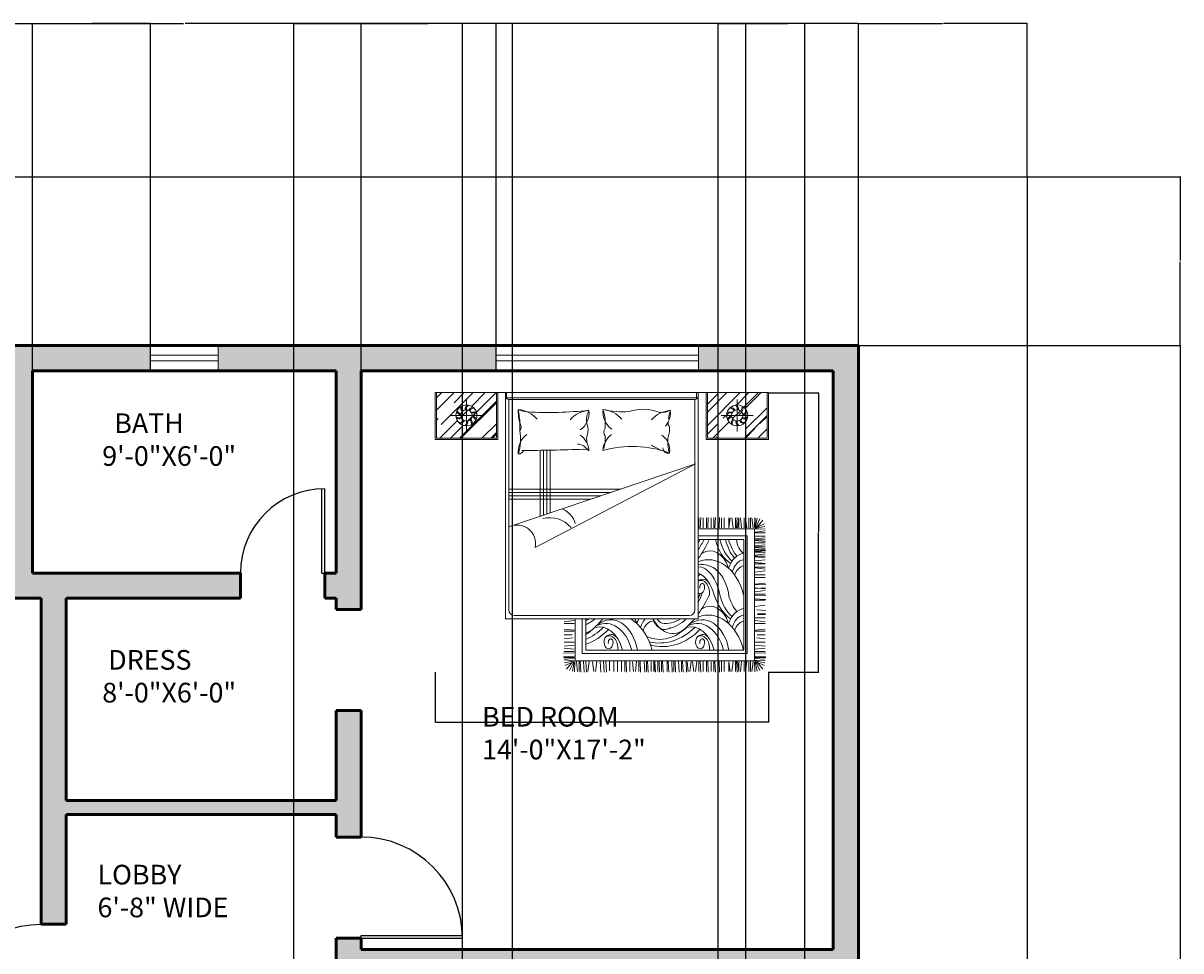
# Model space of a CAD drawing. Units: inches. Extents: x 134045 to 134755, y 144691 to 145880.
# Tile 6 of 6: x 134343 to 134755, y 145550 to 145880. Entities that reach past the tile are written whole.
import ezdxf

# ---------------------------------------------------------------- set-up
doc = ezdxf.new("R2010")
doc.units = ezdxf.units.IN
for name, color, linetype, lineweight in [('A-ANNO-DIMS', 2, 'Continuous', 18), ('A-AREA-IDEN', 7, 'Continuous', 18), ('A-DOOR', 4, 'Continuous', 25), ('A-FURN', 8, 'Continuous', 18), ('A-GLAZ', 4, 'Continuous', 18), ('A-WALL', 7, 'Continuous', 50), ('A-WALL-PATT', 252, 'Continuous', 13), ('C-PROP', 7, 'Continuous', 25)]:
    doc.layers.add(name, color=color, linetype=linetype, lineweight=lineweight)
doc.styles.get("Standard").update_dxf_attribs({"font": 'arial.ttf'})
doc.dimstyles.get("Standard").update_dxf_attribs({"dimtxt": 0.18, "dimasz": 0.18, "dimexe": 0.18, "dimexo": 0.0625, "dimgap": 0.09, "dimtad": 0, "dimtih": 1, "dimtoh": 1, "dimdec": 4, "dimzin": 0, "dimdsep": 46, "dimtxsty": 'Standard', "dimcen": 0.09, "dimadec": 0, "dimazin": 0, "dimtfac": 1, "dimtdec": 4, "dimtofl": 0, "dimtmove": 0, "dimatfit": 3, "dimfxl": 1, "dimtolj": 1, "dimtzin": 0, "dimarcsym": 0})

# ---------------------------------------------------------------- blocks, each defined once
blk = doc.blocks.new('A$C64B41DC1')
for p, q in [((0, 2.508), (2.99, 2.508)), ((0, 2.088), (0, 2.508)), ((0.012, 2.462), (0.058, 2.508)), ((0.012, 2.352), (0.168, 2.508)), ((0.012, 2.1), (0.012, 2.508)), ((0.054, 2.221), (0.341, 2.508)), ((0.169, 2.418), (0.259, 2.508)), ((0.327, 2.386), (0.448, 2.508)), ((0.37, 2.333), (0.545, 2.508)), ((0.548, 2.508), (0.548, 2.1)), ((0.56, 2.508), (0.56, 2.088)), ((0.63, 2.508), (0.63, 0.478)), ((0.64, 2.461), (0.64, 2.508)), ((0.64, 2.508), (2.344, 2.508)), ((2.344, 2.508), (2.36, 2.508)), ((2.344, 2.508), (2.344, 2.461)), ((2.36, 2.508), (2.36, 2.476)), ((2.36, 0.478), (2.36, 2.508)), ((2.43, 2.508), (2.43, 2.088)), ((2.442, 2.508), (2.442, 2.1)), ((2.442, 2.333), (2.617, 2.508)), ((2.442, 2.214), (2.736, 2.508)), ((2.442, 2.404), (2.535, 2.497)), ((2.705, 2.398), (2.815, 2.508)), ((2.769, 2.377), (2.9, 2.508)), ((2.782, 2.365), (2.925, 2.508)), ((2.978, 2.1), (2.978, 2.508)), ((2.99, 2.088), (2.99, 2.508)), ((0.216, 2.1), (0.548, 2.432)), ((0.23, 2.1), (0.548, 2.418)), ((0.28, 2.16), (0.28, 2.448)), ((2.344, 2.461), (0.64, 2.461)), ((0.66, 2.446), (1.495, 2.446)), ((0.66, 2.446), (0.66, 0.558)), ((1.495, 2.446), (0.67, 2.446)), ((2.33, 2.446), (1.495, 2.446)), ((2.33, 0.558), (2.33, 2.446)), ((2.71, 2.16), (2.71, 2.448)), ((0.136, 2.304), (0.425, 2.304)), ((0.231, 2.291), (0.294, 2.353)), ((0.291, 2.254), (0.33, 2.294)), ((0.341, 2.304), (0.36, 2.324)), ((2.854, 2.304), (2.566, 2.304)), ((2.585, 2.278), (2.616, 2.309)), ((2.616, 2.309), (2.631, 2.324)), ((2.667, 2.276), (2.738, 2.346)), ((2.725, 2.308), (2.751, 2.334)), ((2.775, 2.1), (2.978, 2.304)), ((2.791, 2.185), (2.978, 2.371)), ((2.914, 2.231), (2.978, 2.295)), ((0.012, 2.261), (0.027, 2.276)), ((0.04, 2.1), (0.198, 2.258)), ((0.137, 2.1), (0.251, 2.214)), ((0.419, 2.1), (0.548, 2.229)), ((2.442, 2.135), (2.538, 2.231)), ((2.492, 2.1), (2.637, 2.245)), ((2.783, 2.1), (2.868, 2.185)), ((0.56, 2.088), (0, 2.088)), ((0.548, 2.1), (0.012, 2.1)), ((0.499, 2.1), (0.548, 2.149)), ((0.513, 2.1), (0.548, 2.135)), ((2.43, 2.088), (2.99, 2.088)), ((2.442, 2.1), (2.978, 2.1)), ((2.517, 2.1), (2.527, 2.11)), ((2.896, 2.1), (2.978, 2.182)), ((0.942, 1.99), (0.942, 1.397)), ((0.972, 1.991), (0.972, 1.408)), ((1.002, 1.991), (1.002, 1.418)), ((1.032, 1.992), (1.032, 1.428)), ((2.335, 1.868), (0.661, 1.303)), ((0.896, 1.119), (2.335, 1.868)), ((1.664, 1.641), (0.66, 1.641)), ((1.575, 1.611), (0.66, 1.611)), ((2.366, 1.295), (2.366, 1.384)), ((2.377, 1.295), (2.382, 1.389)), ((2.403, 1.295), (2.403, 1.384)), ((2.435, 1.295), (2.435, 1.384)), ((2.445, 1.295), (2.45, 1.389)), ((2.477, 1.296), (2.477, 1.384)), ((2.5, 1.295), (2.5, 1.384)), ((2.51, 1.295), (2.516, 1.389)), ((2.537, 1.295), (2.537, 1.384)), ((2.547, 1.295), (2.552, 1.389)), ((2.568, 1.295), (2.568, 1.384)), ((2.592, 1.295), (2.592, 1.384)), ((2.635, 1.296), (2.635, 1.384)), ((2.636, 1.296), (2.647, 1.384)), ((2.673, 1.295), (2.662, 1.384)), ((2.694, 1.295), (2.694, 1.384)), ((2.704, 1.295), (2.71, 1.389)), ((2.713, 1.296), (2.723, 1.384)), ((2.725, 1.295), (2.725, 1.384)), ((2.749, 1.295), (2.739, 1.384)), ((2.772, 1.295), (2.772, 1.384)), ((2.796, 1.295), (2.785, 1.384)), ((2.815, 1.296), (2.815, 1.384)), ((2.815, 1.296), (2.815, 1.384)), ((2.828, 1.295), (2.828, 1.384)), ((2.828, 1.295), (2.828, 1.384)), ((2.852, 1.295), (2.842, 1.384)), ((2.852, 1.295), (2.842, 1.384)), ((2.865, 1.297), (2.869, 1.386)), ((2.871, 1.296), (2.871, 1.384)), ((2.871, 1.296), (2.888, 1.382)), ((2.877, 1.296), (2.913, 1.376)), ((2.889, 1.301), (2.939, 1.364)), ((2.36, 1.287), (2.864, 1.287)), ((2.864, 1.287), (2.864, 0.102)), ((2.871, 1.293), (2.954, 1.332)), ((2.872, 1.288), (2.959, 1.306)), ((2.872, 1.256), (2.96, 1.267)), ((2.872, 1.249), (2.96, 1.249)), ((2.874, 1.282), (2.96, 1.287)), ((2.36, 1.223), (2.8, 1.223)), ((2.36, 1.191), (2.768, 1.191)), ((2.768, 1.191), (2.768, 0.198)), ((2.8, 1.223), (2.8, 0.166)), ((2.872, 1.221), (2.96, 1.221)), ((2.872, 1.195), (2.96, 1.205)), ((2.872, 1.187), (2.96, 1.187)), ((2.872, 1.181), (2.96, 1.171)), ((2.872, 1.159), (2.96, 1.159)), ((2.872, 1.133), (2.96, 1.143)), ((2.872, 1.125), (2.96, 1.125)), ((2.872, 1.119), (2.96, 1.109)), ((2.872, 1.104), (2.96, 1.093)), ((2.872, 1.097), (2.96, 1.097)), ((2.872, 1.086), (2.966, 1.091)), ((2.872, 1.086), (2.96, 1.075)), ((2.872, 1.076), (2.96, 1.076)), ((2.872, 1.049), (2.96, 1.06)), ((2.872, 1.042), (2.96, 1.042)), ((2.872, 1.035), (2.96, 1.025)), ((2.872, 0.999), (2.96, 1.009)), ((2.872, 0.985), (2.96, 0.974)), ((2.872, 0.973), (2.96, 0.973)), ((2.872, 0.941), (2.96, 0.941)), ((2.872, 0.935), (2.96, 0.924)), ((2.872, 0.898), (2.96, 0.908)), ((2.872, 0.873), (2.96, 0.873)), ((2.872, 0.85), (2.96, 0.85)), ((2.872, 0.789), (2.96, 0.799)), ((2.872, 0.782), (2.966, 0.787)), ((2.872, 0.757), (2.96, 0.747)), ((2.872, 0.75), (2.966, 0.756)), ((2.872, 0.72), (2.96, 0.731)), ((2.872, 0.699), (2.96, 0.699)), ((2.872, 0.689), (2.966, 0.684)), ((2.872, 0.658), (2.966, 0.652)), ((2.872, 0.647), (2.96, 0.647)), ((2.872, 0.59), (2.96, 0.601)), ((2.882, 0.558), (2.966, 0.554)), ((2.891, 0.526), (2.966, 0.522)), ((0.63, 0.478), (2.36, 0.478)), ((0.71, 0.508), (2.28, 0.508)), ((1.246, 0.463), (1.158, 0.452)), ((1.246, 0.437), (1.158, 0.437)), ((1.254, 0.102), (1.254, 0.478)), ((1.318, 0.166), (1.318, 0.478)), ((1.35, 0.198), (1.35, 0.478)), ((2.872, 0.488), (2.96, 0.488)), ((2.872, 0.463), (2.96, 0.452)), ((2.872, 0.437), (2.96, 0.437)), ((2.893, 0.517), (2.96, 0.517)), ((1.246, 0.375), (1.158, 0.385)), ((1.246, 0.368), (1.158, 0.368)), ((1.229, 0.336), (1.158, 0.336)), ((2.872, 0.375), (2.96, 0.385)), ((2.872, 0.368), (2.96, 0.368)), ((2.89, 0.336), (2.96, 0.336)), ((1.235, 0.309), (1.158, 0.3)), ((1.246, 0.268), (1.158, 0.268)), ((1.246, 0.242), (1.158, 0.232)), ((1.246, 0.206), (1.158, 0.216)), ((2.872, 0.268), (2.96, 0.268)), ((2.872, 0.242), (2.96, 0.232)), ((2.872, 0.206), (2.96, 0.216)), ((2.883, 0.309), (2.96, 0.3)), ((1.246, 0.174), (1.152, 0.169)), ((1.246, 0.143), (1.152, 0.138)), ((1.246, 0.133), (1.152, 0.128)), ((1.246, 0.185), (1.158, 0.185)), ((1.246, 0.132), (1.158, 0.132)), ((1.246, 0.132), (1.158, 0.132)), ((1.246, 0.1), (1.158, 0.11)), ((1.246, 0.123), (1.159, 0.117)), ((2.8, 0.166), (1.318, 0.166)), ((2.768, 0.198), (1.35, 0.198)), ((2.872, 0.185), (2.96, 0.185)), ((2.872, 0.174), (2.966, 0.169)), ((2.872, 0.143), (2.966, 0.138)), ((2.872, 0.133), (2.966, 0.128)), ((2.872, 0.132), (2.96, 0.132)), ((2.872, 0.123), (2.959, 0.117)), ((2.874, 0.107), (2.96, 0.102)), ((1.246, 0.101), (1.159, 0.083)), ((1.247, 0.096), (1.164, 0.058)), ((1.229, 0.088), (1.179, 0.026)), ((1.242, 0.093), (1.205, 0.013)), ((1.247, 0.093), (1.231, 0.007)), ((1.253, 0.092), (1.249, 0.003)), ((2.864, 0.102), (1.254, 0.102)), ((1.266, 0.094), (1.276, 0.005)), ((1.29, 0.094), (1.29, 0.005)), ((1.3, 0.094), (1.305, 0)), ((1.331, 0.094), (1.337, 0)), ((1.352, 0.094), (1.358, 0)), ((1.38, 0.094), (1.37, 0.005)), ((1.412, 0.093), (1.422, 0.005)), ((1.449, 0.094), (1.438, 0.005)), ((1.48, 0.094), (1.485, 0)), ((1.511, 0.094), (1.517, 0)), ((1.532, 0.094), (1.538, 0)), ((1.564, 0.094), (1.564, 0.01)), ((1.602, 0.094), (1.602, 0.005)), ((1.634, 0.094), (1.634, 0.005)), ((1.67, 0.094), (1.67, 0.005)), ((1.702, 0.094), (1.702, 0.005)), ((1.712, 0.094), (1.717, 0)), ((1.745, 0.093), (1.745, 0.005)), ((1.77, 0.093), (1.78, 0.005)), ((1.806, 0.094), (1.796, 0.005)), ((1.827, 0.094), (1.827, 0.005)), ((1.838, 0.094), (1.843, 0)), ((1.875, 0.094), (1.88, 0)), ((1.896, 0.094), (1.896, 0.005)), ((1.906, 0.094), (1.911, 0)), ((1.938, 0.093), (1.938, 0.005)), ((1.961, 0.094), (1.961, 0.005)), ((1.964, 0.093), (1.974, 0.005)), ((1.971, 0.094), (1.977, 0)), ((1.998, 0.094), (1.998, 0.005)), ((2.008, 0.094), (2.013, 0)), ((2.029, 0.094), (2.029, 0.005)), ((2.039, 0.094), (2.045, 0)), ((2.08, 0.094), (2.08, 0.005)), ((2.09, 0.094), (2.095, 0)), ((2.122, 0.094), (2.127, 0)), ((2.141, 0.094), (2.141, 0.005)), ((2.152, 0.094), (2.157, 0)), ((2.183, 0.094), (2.188, 0)), ((2.209, 0.094), (2.209, 0.005)), ((2.22, 0.094), (2.225, 0)), ((2.251, 0.094), (2.256, 0)), ((2.26, 0.093), (2.271, 0.005)), ((2.297, 0.094), (2.286, 0.005)), ((2.309, 0.093), (2.319, 0.005)), ((2.346, 0.094), (2.335, 0.005)), ((2.366, 0.094), (2.366, 0.005)), ((2.377, 0.094), (2.382, 0)), ((2.403, 0.094), (2.403, 0.005)), ((2.435, 0.094), (2.435, 0.005)), ((2.445, 0.094), (2.45, 0)), ((2.477, 0.093), (2.477, 0.005)), ((2.5, 0.094), (2.5, 0.005)), ((2.51, 0.094), (2.516, 0)), ((2.537, 0.094), (2.537, 0.005)), ((2.547, 0.094), (2.552, 0)), ((2.568, 0.094), (2.568, 0.005)), ((2.592, 0.094), (2.592, 0.005)), ((2.635, 0.093), (2.635, 0.005)), ((2.636, 0.093), (2.647, 0.005)), ((2.673, 0.094), (2.662, 0.005)), ((2.694, 0.094), (2.694, 0.005)), ((2.704, 0.094), (2.71, 0)), ((2.713, 0.093), (2.723, 0.005)), ((2.725, 0.094), (2.725, 0.005)), ((2.749, 0.094), (2.739, 0.005)), ((2.772, 0.094), (2.772, 0.005)), ((2.796, 0.094), (2.785, 0.005)), ((2.815, 0.093), (2.815, 0.005)), ((2.828, 0.094), (2.828, 0.005)), ((2.852, 0.094), (2.842, 0.005)), ((2.865, 0.092), (2.869, 0.003)), ((2.871, 0.096), (2.954, 0.058)), ((2.871, 0.093), (2.888, 0.007)), ((2.872, 0.101), (2.959, 0.083)), ((2.877, 0.093), (2.913, 0.013)), ((2.889, 0.088), (2.939, 0.026))]:
    blk.add_line(p, q)
at = {"ltscale": 10}
for p, q in [((1.486, 1.581), (0.66, 1.581)), ((1.397, 1.551), (0.66, 1.551))]:
    blk.add_line(p, q, dxfattribs=at)
for centre, radius in [((0.28, 2.304), 0.0942), ((2.71, 2.304), 0.0942), ((0.28, 2.304), 0.051), ((2.71, 2.304), 0.051)]:
    blk.add_circle(centre, radius)
for centre, radius, start, end in [((0.329, 2.356), 0.0605, 136.17, 182.4897), ((0.323, 2.358), 0.0462, 124.3002, 184.538), ((0.66, 2.476), 0.03, 180, 270), ((2.33, 2.476), 0.03, 270, 0), ((2.667, 2.358), 0.0462, 355.462, 55.6998), ((2.662, 2.356), 0.0605, 357.5103, 43.83), ((0.215, 2.328), 0.0462, 232.3002, 292.538), ((0.246, 2.366), 0.0605, 208.17, 254.4897), ((0.242, 2.361), 0.0462, 196.3002, 256.538), ((0.289, 2.374), 0.0605, 172.17, 218.4897), ((0.283, 2.373), 0.0462, 160.3002, 220.538), ((0.35, 2.318), 0.0605, 100.17, 146.4897), ((0.347, 2.323), 0.0462, 88.3002, 148.538), ((0.345, 2.274), 0.0605, 64.17, 110.4897), ((0.345, 2.28), 0.0462, 52.3002, 112.538), ((0.319, 2.246), 0.0462, 16.3002, 76.538), ((0.315, 2.242), 0.0605, 28.17, 74.4897), ((1.053, 2.33), 0.308, 175.3048, 198.6942), ((-0.87, 2.094), 1.636, 4.8098, 9.1892), ((0.858, 2.628), 0.295, 247.5179, 264.267), ((0.728, 2.111), 0.245, 40.4189, 85.9871), ((1.016, 5.71), 3.38, 266.8134, 276.1602), ((1.396, 2.104), 0.245, 94.0129, 139.5811), ((1.186, 2.329), 0.194, 306.5711, 5.89), ((1.535, 2.265), 0.177, 151.7736, 201.6983), ((1.699, 2.335), 0.194, 174.11, 233.4289), ((1.148, 2.231), 0.378, 353.4947, 19.1867), ((1.687, 3.192), 0.856, 257.7438, 273.6284), ((1.488, 2.111), 0.245, 40.4189, 85.9871), ((1.867, 1.971), 0.388, 68.2026, 108.9817), ((2.127, 2.104), 0.245, 94.0129, 139.5811), ((2.034, 2.486), 0.156, 261.5958, 298.9092), ((1.916, 2.329), 0.194, 333.7371, 5.89), ((2.606, 2.203), 0.517, 163.6046, 172.3273), ((2.645, 2.28), 0.0462, 67.462, 127.6998), ((2.645, 2.274), 0.0605, 69.5103, 115.83), ((2.675, 2.242), 0.0605, 105.5103, 151.83), ((2.671, 2.246), 0.0462, 103.462, 163.6998), ((2.643, 2.323), 0.0462, 31.462, 91.6998), ((2.64, 2.318), 0.0605, 33.5103, 79.83), ((2.707, 2.373), 0.0462, 319.462, 19.6998), ((2.702, 2.374), 0.0605, 321.5103, 7.83), ((2.775, 2.328), 0.0462, 247.462, 307.6998), ((2.749, 2.361), 0.0462, 283.462, 343.6998), ((2.745, 2.366), 0.0605, 285.5103, 331.83), ((0.216, 2.334), 0.0605, 244.17, 290.4897), ((0.214, 2.285), 0.0462, 268.3002, 328.538), ((0.211, 2.29), 0.0605, 280.17, 326.4897), ((0.238, 2.249), 0.0462, 304.3002, 4.538), ((0.232, 2.252), 0.0605, 316.17, 2.4897), ((0.278, 2.235), 0.0462, 340.3002, 40.538), ((0.272, 2.233), 0.0605, 352.17, 38.4897), ((0.727, 2.201), 0.0446, 314.4736, 42.1713), ((-1.601, 2.277), 2.362, 357.3905, 358.8876), ((1.204, 2.178), 0.168, 337.017, 7.5368), ((1.567, 2.155), 0.0547, 142.0833, 220.902), ((1.916, 2.329), 0.194, 320.9404, 333.7371), ((2.135, 2.231), 0.0459, 165.3506, 223.2684), ((1.935, 2.178), 0.168, 337.017, 7.5368), ((2.718, 2.233), 0.0605, 141.5103, 187.83), ((2.712, 2.235), 0.0462, 139.462, 199.6998), ((2.758, 2.252), 0.0605, 177.5103, 223.83), ((2.753, 2.249), 0.0462, 175.462, 235.6998), ((2.78, 2.29), 0.0605, 213.5103, 259.83), ((2.777, 2.285), 0.0462, 211.462, 271.6998), ((2.774, 2.334), 0.0605, 249.5103, 295.83), ((0.938, 1.978), 0.194, 126.5711, 185.89), ((0.269, 2.094), 0.496, 344.0243, 8.7071), ((1.186, 1.971), 0.194, 4.3181, 53.4289), ((1.541, 2.097), 0.183, 175.2233, 196.23), ((1.706, 1.971), 0.204, 127.1197, 175.09), ((1.196, 2.098), 0.33, 343.7954, 3.5554), ((1.939, 1.991), 0.165, 351.2621, 55.7572), ((2.462, 2.072), 0.375, 173.8296, 196.4356), ((0.742, 2.015), 0.057, 273.4709, 328.5412), ((0.725, 18.844), 16.855, 270.174, 272.0521), ((1.269, 1.925), 0.122, 33.628, 86.4744), ((1.34, 1.94), 0.0603, 49.0991, 101.3702), ((1.768, 1.063), 0.963, 69.6507, 105.9631), ((2.275, 2.579), 0.637, 238.3499, 254.3137), ((2.091, 2.012), 0.0478, 179.7727, 283.8018), ((0.728, 2.202), 0.245, 274.0129, 278.3417), ((1.075, 1.287), 0.187, 14.1863, 69.1212), ((1.027, 1.133), 0.253, 40.629, 104.3712), ((0.735, 1.155), 0.165, 347.3109, 116.4454), ((0.71, 0.558), 0.05, 180, 270), ((2.28, 0.558), 0.05, 270, 0)]:
    blk.add_arc(centre, radius, start, end)
for centre, major_axis, ratio, start_param, end_param in [((1.994, 1.626), (0, -0.753), 0.68, 0.797284, 0.954936), ((2.064, 1.466), (0, -0.532), 0.68, 7.239912, 7.311536), ((1.905, 1.74), (0, -0.984), 0.68, 0.74745, 0.979724), ((2.746, 1.308), (0, 0.361), 0.68, 1.900046, 2.742661), ((2.787, 1.308), (0, 0.361), 0.68, 1.900046, 2.614747), ((2.837, 1.308), (0, 0.361), 0.68, 1.900046, 2.479658), ((2.861, 1.321), (0, 0.361), 0.68, 1.938265, 2.479658), ((2.806, 1.208), (0, -0.152), 0.68, 4.821745, 5.895886), ((2.451, 0.507), (0, 0.502), 0.68, 5.095327, 6.553458), ((2.467, 0.822), (0, -0.266), 0.68, 2.006169, 3.565187), ((2.786, 0.807), (0, -0.261), 0.68, 3.244645, 4.205018), ((2.396, 0.603), (0, 0.364), 0.68, -1.3172, 0.145284), ((2.351, 0.564), (0.007, 0.382), 0.56205, -1.21172, -0.009991), ((2.778, 0.829), (0, -0.18), 0.68, 3.227058, 4.318474), ((2.782, 0.797), (0, -0.159), 0.68, 3.272942, 4.229533), ((2.296, 0.577), (0, -0.326), 0.68, 1.938944, 2.850232), ((2.04, 1.601), (0, -0.876), 0.68, 6.849801, 6.887077), ((2.4, 0.713), (0, -0.121), 0.68, 2.284368, 3.652258), ((2.383, 0.708), (0, 0.115), 0.68, 4.593909, 6.585576), ((2.377, 0.765), (0, -0.0593), 0.68, 5.841311, 7.755362), ((2.396, 0.763), (0, -0.0317), 0.68, 1.462497, 5.046281), ((1.994, 1.13), (-0.068, 0.744), 0.610498, 3.917146, 4.063997), ((2.064, 0.969), (0, -0.532), 0.68, 7.239912, 7.336618), ((1.905, 1.243), (0, -0.984), 0.68, 0.74745, 0.979724), ((2.467, 0.325), (0, -0.266), 0.68, 2.006169, 3.565187), ((2.746, 0.811), (-0.06, 0.373), 0.695517, 1.775813, 2.548612), ((2.787, 0.811), (0, 0.361), 0.68, 1.900046, 2.614747), ((2.861, 0.824), (0, 0.361), 0.68, 1.938265, 2.479658), ((2.451, 0.01), (0, 0.502), 0.68, 5.095327, 6.553458), ((2.786, 0.31), (0, -0.261), 0.68, 3.244645, 4.205018), ((1.242, 0.969), (0, -0.532), 0.68, 6.586764, 6.677612), ((1.171, 1.13), (-0.116, 0.724), 0.59432, 3.291697, 3.50733), ((1.474, 0.08), (0, -0.326), 0.68, 1.938944, 3.339184), ((1.083, 1.243), (0, -0.984), 0.68, 0.565948, 0.680366), ((1.528, 0.067), (0, -0.37), 0.68, 1.930561, 3.464283), ((1.574, 0.106), (0, 0.364), 0.68, -1.3172, 0.476403), ((1.629, 0.01), (0, 0.502), 0.68, 6.655152, 6.661293), ((1.629, 0.01), (0, 0.502), 0.68, 5.095327, 5.911219), ((1.644, 0.325), (0, -0.266), 0.68, 2.006169, 2.182797), ((1.964, 0.31), (0, -0.261), 0.68, 4.015924, 4.205018), ((1.956, 0.332), (0, -0.18), 0.68, 3.770744, 4.318474), ((1.96, 0.3), (0, -0.159), 0.68, 3.14258, 4.229533), ((2.061, 0.562), (0, -0.18), 0.68, 5.194792, 5.929328), ((2.061, 0.562), (0, -0.18), 0.68, 5.194792, 6.723255), ((2.131, 0.66), (0, -0.315), 0.68, 5.328638, 6.949396), ((2.055, 0.566), (0, -0.13), 0.68, 5.450951, 6.054641), ((2.064, 0.969), (0, -0.532), 0.68, 6.20013, 6.677612), ((1.994, 1.13), (-0.068, 0.744), 0.610498, 3.199135, 3.592282), ((2.296, 0.08), (0, -0.326), 0.68, 1.938944, 3.339184), ((1.905, 1.243), (0, -0.984), 0.68, 0.565948, 0.680366), ((2.351, 0.067), (0, -0.37), 0.68, 1.930561, 3.464283), ((2.396, 0.106), (0, 0.364), 0.68, -1.3172, 0.476403), ((2.451, 0.01), (0, 0.502), 0.68, 6.655152, 6.661293), ((2.778, 0.332), (0, -0.18), 0.68, 3.227058, 4.318474), ((2.782, 0.3), (0, -0.159), 0.68, 3.272942, 4.229533), ((1.193, 0.918), (0, -0.624), 0.68, 0.378672, 0.625379), ((1.309, 0.66), (0, -0.315), 0.68, 6.475719, 6.949396), ((1.191, 1.107), (0, 0.846), 0.68, 3.421828, 3.728616), ((1.218, 1.105), (0, -0.876), 0.68, 6.507006, 6.887077), ((1.555, 0.269), (0, -0.0593), 0.68, 3.732151, 7.755362), ((1.578, 0.217), (0, -0.121), 0.68, 2.284368, 3.726131), ((1.561, 0.211), (0, 0.115), 0.68, 4.593909, 6.647252), ((2.016, 0.918), (0, -0.624), 0.68, -0.280078, 0.625379), ((2.013, 1.107), (0, 0.846), 0.68, 2.978727, 3.728616), ((2.04, 1.105), (0, -0.876), 0.68, 6.099302, 6.887077), ((2.377, 0.269), (0, -0.0593), 0.68, 3.732151, 7.755362), ((2.4, 0.217), (0, -0.121), 0.68, 2.284368, 3.726131), ((2.383, 0.211), (0, 0.115), 0.68, 4.593909, 6.647252), ((1.574, 0.266), (0, -0.0317), 0.68, 1.462497, 5.046281), ((2.396, 0.266), (0, -0.0317), 0.68, 1.462497, 5.046281)]:
    blk.add_ellipse(centre, major_axis=major_axis, ratio=ratio, start_param=start_param, end_param=end_param)
blk = doc.blocks.new('DOOR-SWING-36IN')
for p, q in [((0, 1), (35.99, 1)), ((0, 0), (0, 1)), ((0, 0), (36, 0))]:
    blk.add_line(p, q)
blk.add_arc((0, 0), 36, 0, 90)
blk = doc.blocks.new('DOOR-SWING-30IN')
for p, q in [((0, 1), (29.98, 1)), ((0, 1), (0, 0)), ((0, 0), (30, 0))]:
    blk.add_line(p, q)
blk.add_arc((0, 0), 30, 0, 90)
blk = doc.blocks.new('WIN-GLAZ-24IN')
for p, q in [((0, 0), (0, 24)), ((2, 0), (2, 24))]:
    blk.add_line(p, q)
blk = doc.blocks.new('WIN-GLAZ-72IN')
for p, q in [((0, 72), (0, 0)), ((2, 72), (2, 0))]:
    blk.add_line(p, q)
blk = doc.blocks.new('*D32')
at = {"layer": 'A-ANNO-DIMS', "color": 0, "lineweight": -2, "transparency": 16777216}
for p, q in [((134489.45, 145649.04), (134489.45, 145631.13)), ((134608.05, 145649.04), (134608.05, 145631.13)), ((134489.63, 145631.31), (134547.37, 145631.31)), ((134607.87, 145631.31), (134550.14, 145631.31))]:
    blk.add_line(p, q, dxfattribs=at)
at = {"layer": 'A-ANNO-DIMS', "color": 0, "transparency": 16777216}
for points in [[(134489.63, 145631.34), (134489.63, 145631.28), (134489.45, 145631.31)], [(134607.87, 145631.34), (134607.87, 145631.28), (134608.05, 145631.31)]]:
    blk.add_solid(points, dxfattribs=at)
at = {"layer": 'Defpoints', "color": 0, "transparency": 16777216}
for p in [(134489.45, 145649.1), (134608.05, 145649.1), (134608.05, 145631.31)]:
    blk.add_point(p, dxfattribs=at)
at = {"layer": 'A-ANNO-DIMS', "color": 0, "transparency": 16777216, "insert": (134548.75, 145631.31), "char_height": 0.18, "attachment_point": 5}
blk.add_mtext('\\A1;BED GROUP 119 TYP.', dxfattribs=at)
blk = doc.blocks.new('*D33')
at = {"layer": 'A-ANNO-DIMS', "color": 0, "lineweight": -2, "transparency": 16777216}
for p, q in [((134608.12, 145748.57), (134626.03, 145748.57)), ((134625.85, 145748.39), (134625.85, 145699.02)), ((134625.85, 145649.28), (134625.85, 145698.65)), ((134608.12, 145649.1), (134626.03, 145649.1))]:
    blk.add_line(p, q, dxfattribs=at)
at = {"layer": 'A-ANNO-DIMS', "color": 0, "transparency": 16777216}
for points in [[(134625.82, 145748.39), (134625.88, 145748.39), (134625.85, 145748.57)], [(134625.82, 145649.28), (134625.88, 145649.28), (134625.85, 145649.1)]]:
    blk.add_solid(points, dxfattribs=at)
at = {"layer": 'Defpoints', "color": 0, "transparency": 16777216}
for p in [(134608.05, 145748.57), (134625.85, 145748.57), (134608.05, 145649.1)]:
    blk.add_point(p, dxfattribs=at)
at = {"layer": 'A-ANNO-DIMS', "color": 0, "transparency": 16777216, "insert": (134625.85, 145698.83), "char_height": 0.18, "attachment_point": 5}
blk.add_mtext('\\A1;99 TYP.', dxfattribs=at)
blk = doc.blocks.new('*D48')
at = {"layer": 'A-ANNO-DIMS', "color": 0, "lineweight": -2, "transparency": 16777216}
for p, q in [((134160.1, 145765.44), (134160.1, 145880.11)), ((134160.28, 145879.93), (134399.81, 145879.93)), ((134639.92, 145879.93), (134400.4, 145879.93)), ((134640.1, 145765.44), (134640.1, 145880.11))]:
    blk.add_line(p, q, dxfattribs=at)
at = {"layer": 'A-ANNO-DIMS', "color": 0, "transparency": 16777216}
for points in [[(134160.28, 145879.96), (134160.28, 145879.9), (134160.1, 145879.93)], [(134639.92, 145879.96), (134639.92, 145879.9), (134640.1, 145879.93)]]:
    blk.add_solid(points, dxfattribs=at)
at = {"layer": 'Defpoints', "color": 0, "transparency": 16777216}
for p in [(134640.1, 145879.93), (134160.1, 145765.38), (134640.1, 145765.38)]:
    blk.add_point(p, dxfattribs=at)
at = {"layer": 'A-ANNO-DIMS', "color": 0, "transparency": 16777216, "insert": (134400.1, 145879.93), "char_height": 0.18, "attachment_point": 5}
blk.add_mtext('\\A1;480', dxfattribs=at)
blk = doc.blocks.new('*D49')
at = {"layer": 'A-ANNO-DIMS', "color": 0, "lineweight": -2, "transparency": 16777216}
for p, q in [((134640.17, 145765.38), (134754.83, 145765.38)), ((134754.65, 145765.2), (134754.65, 145358.06)), ((134754.65, 144950.56), (134754.65, 145357.69)), ((134640.17, 144950.38), (134754.83, 144950.38))]:
    blk.add_line(p, q, dxfattribs=at)
at = {"layer": 'A-ANNO-DIMS', "color": 0, "transparency": 16777216}
for points in [[(134754.62, 145765.2), (134754.68, 145765.2), (134754.65, 145765.38)], [(134754.62, 144950.56), (134754.68, 144950.56), (134754.65, 144950.38)]]:
    blk.add_solid(points, dxfattribs=at)
at = {"layer": 'Defpoints', "color": 0, "transparency": 16777216}
for p in [(134640.1, 145765.38), (134754.65, 145765.38), (134640.1, 144950.38)]:
    blk.add_point(p, dxfattribs=at)
at = {"layer": 'A-ANNO-DIMS', "color": 0, "transparency": 16777216, "insert": (134754.65, 145357.88), "char_height": 0.18, "attachment_point": 5}
blk.add_mtext('\\A1;815', dxfattribs=at)
blk = doc.blocks.new('*D51')
at = {"layer": 'A-ANNO-DIMS', "color": 0, "lineweight": -2, "transparency": 16777216}
for p, q in [((134640.1, 145765.44), (134640.1, 145880.11)), ((134640.28, 145879.93), (134669.88, 145879.93)), ((134699.92, 145879.93), (134670.32, 145879.93)), ((134700.1, 145825.44), (134700.1, 145880.11))]:
    blk.add_line(p, q, dxfattribs=at)
at = {"layer": 'A-ANNO-DIMS', "color": 0, "transparency": 16777216}
for points in [[(134640.28, 145879.96), (134640.28, 145879.9), (134640.1, 145879.93)], [(134699.92, 145879.96), (134699.92, 145879.9), (134700.1, 145879.93)]]:
    blk.add_solid(points, dxfattribs=at)
at = {"layer": 'Defpoints', "color": 0, "transparency": 16777216}
for p in [(134700.1, 145879.93), (134700.1, 145825.38), (134640.1, 145765.38)]:
    blk.add_point(p, dxfattribs=at)
at = {"layer": 'A-ANNO-DIMS', "color": 0, "transparency": 16777216, "insert": (134670.1, 145879.93), "char_height": 0.18, "attachment_point": 5}
blk.add_mtext('\\A1;60', dxfattribs=at)
blk = doc.blocks.new('*D52')
at = {"layer": 'A-ANNO-DIMS', "color": 0, "lineweight": -2, "transparency": 16777216}
for p, q in [((134700.17, 145825.38), (134754.83, 145825.38)), ((134754.65, 145825.2), (134754.65, 145795.56)), ((134754.65, 145765.56), (134754.65, 145795.19)), ((134640.17, 145765.38), (134754.83, 145765.38))]:
    blk.add_line(p, q, dxfattribs=at)
at = {"layer": 'A-ANNO-DIMS', "color": 0, "transparency": 16777216}
for points in [[(134754.62, 145825.2), (134754.68, 145825.2), (134754.65, 145825.38)], [(134754.62, 145765.56), (134754.68, 145765.56), (134754.65, 145765.38)]]:
    blk.add_solid(points, dxfattribs=at)
at = {"layer": 'Defpoints', "color": 0, "transparency": 16777216}
for p in [(134700.1, 145825.38), (134640.1, 145765.38), (134754.65, 145765.38)]:
    blk.add_point(p, dxfattribs=at)
at = {"layer": 'A-ANNO-DIMS', "color": 0, "transparency": 16777216, "insert": (134754.65, 145795.38), "char_height": 0.18, "attachment_point": 5}
blk.add_mtext('\\A1;60', dxfattribs=at)
blk = doc.blocks.new('*D57')
at = {"layer": 'A-ANNO-DIMS', "color": 0, "lineweight": -2, "transparency": 16777216}
for p, q in [((134590.1, 145259.44), (134590.1, 145880.11)), ((134590.28, 145879.93), (134614.89, 145879.93)), ((134639.92, 145879.93), (134615.32, 145879.93)), ((134640.1, 145259.44), (134640.1, 145880.11))]:
    blk.add_line(p, q, dxfattribs=at)
at = {"layer": 'A-ANNO-DIMS', "color": 0, "transparency": 16777216}
for points in [[(134590.28, 145879.96), (134590.28, 145879.9), (134590.1, 145879.93)], [(134639.92, 145879.96), (134639.92, 145879.9), (134640.1, 145879.93)]]:
    blk.add_solid(points, dxfattribs=at)
at = {"layer": 'Defpoints', "color": 0, "transparency": 16777216}
for p in [(134590.1, 145879.93), (134590.1, 145259.38), (134640.1, 145259.38)]:
    blk.add_point(p, dxfattribs=at)
at = {"layer": 'A-ANNO-DIMS', "color": 0, "transparency": 16777216, "insert": (134615.1, 145879.93), "char_height": 0.18, "attachment_point": 5}
blk.add_mtext('\\A1;50', dxfattribs=at)
blk = doc.blocks.new('*D58')
at = {"layer": 'A-ANNO-DIMS', "color": 0, "lineweight": -2, "transparency": 16777216}
for p, q in [((134600.01, 145247.44), (134600.01, 145880.11)), ((134600.19, 145879.93), (134610.3, 145879.93)), ((134620.83, 145879.93), (134610.71, 145879.93)), ((134621.01, 145247.44), (134621.01, 145880.11))]:
    blk.add_line(p, q, dxfattribs=at)
at = {"layer": 'A-ANNO-DIMS', "color": 0, "transparency": 16777216}
for points in [[(134600.19, 145879.96), (134600.19, 145879.9), (134600.01, 145879.93)], [(134620.83, 145879.96), (134620.83, 145879.9), (134621.01, 145879.93)]]:
    blk.add_solid(points, dxfattribs=at)
at = {"layer": 'Defpoints', "color": 0, "transparency": 16777216}
for p in [(134621.01, 145879.93), (134600.01, 145247.37), (134621.01, 145247.37)]:
    blk.add_point(p, dxfattribs=at)
at = {"layer": 'A-ANNO-DIMS', "color": 0, "transparency": 16777216, "insert": (134610.51, 145879.93), "char_height": 0.18, "attachment_point": 5}
blk.add_mtext('\\A1;21', dxfattribs=at)
blk = doc.blocks.new('*D60')
at = {"layer": 'A-ANNO-DIMS', "color": 0, "lineweight": -2, "transparency": 16777216}
for p, q in [((134439.1, 145268.44), (134439.1, 145880.11)), ((134439.28, 145879.93), (134468.88, 145879.93)), ((134498.92, 145879.93), (134469.32, 145879.93)), ((134499.1, 145328.44), (134499.1, 145880.11))]:
    blk.add_line(p, q, dxfattribs=at)
at = {"layer": 'A-ANNO-DIMS', "color": 0, "transparency": 16777216}
for points in [[(134439.28, 145879.96), (134439.28, 145879.9), (134439.1, 145879.93)], [(134498.92, 145879.96), (134498.92, 145879.9), (134499.1, 145879.93)]]:
    blk.add_solid(points, dxfattribs=at)
at = {"layer": 'Defpoints', "color": 0, "transparency": 16777216}
for p in [(134499.1, 145879.93), (134499.1, 145328.38), (134439.1, 145268.38)]:
    blk.add_point(p, dxfattribs=at)
at = {"layer": 'A-ANNO-DIMS', "color": 0, "transparency": 16777216, "insert": (134469.1, 145879.93), "char_height": 0.18, "attachment_point": 5}
blk.add_mtext('\\A1;60', dxfattribs=at)
blk = doc.blocks.new('*D66')
at = {"layer": 'A-ANNO-DIMS', "color": 0, "lineweight": -2, "transparency": 16777216}
for p, q in [((134439.1, 144959.44), (134439.1, 145880.11)), ((134439.28, 145879.93), (134477.68, 145879.93)), ((134516.72, 145879.93), (134478.32, 145879.93)), ((134516.9, 144959.44), (134516.9, 145880.11))]:
    blk.add_line(p, q, dxfattribs=at)
at = {"layer": 'A-ANNO-DIMS', "color": 0, "transparency": 16777216}
for points in [[(134439.28, 145879.96), (134439.28, 145879.9), (134439.1, 145879.93)], [(134516.72, 145879.96), (134516.72, 145879.9), (134516.9, 145879.93)]]:
    blk.add_solid(points, dxfattribs=at)
at = {"layer": 'Defpoints', "color": 0, "transparency": 16777216}
for p in [(134516.9, 145879.93), (134439.1, 144959.38), (134516.9, 144959.38)]:
    blk.add_point(p, dxfattribs=at)
at = {"layer": 'A-ANNO-DIMS', "color": 0, "transparency": 16777216, "insert": (134478, 145879.93), "char_height": 0.18, "attachment_point": 5}
blk.add_mtext('\\A1;77.8', dxfattribs=at)
blk = doc.blocks.new('*D69')
at = {"layer": 'A-ANNO-DIMS', "color": 0, "lineweight": -2, "transparency": 16777216}
for p, q in [((134346.1, 145756.44), (134346.1, 145880.11)), ((134346.28, 145879.93), (134366.88, 145879.93)), ((134387.92, 145879.93), (134367.33, 145879.93)), ((134388.1, 145756.44), (134388.1, 145880.11))]:
    blk.add_line(p, q, dxfattribs=at)
at = {"layer": 'A-ANNO-DIMS', "color": 0, "transparency": 16777216}
for points in [[(134346.28, 145879.96), (134346.28, 145879.9), (134346.1, 145879.93)], [(134387.92, 145879.96), (134387.92, 145879.9), (134388.1, 145879.93)]]:
    blk.add_solid(points, dxfattribs=at)
at = {"layer": 'Defpoints', "color": 0, "transparency": 16777216}
for p in [(134388.1, 145879.93), (134346.1, 145756.38), (134388.1, 145756.38)]:
    blk.add_point(p, dxfattribs=at)
at = {"layer": 'A-ANNO-DIMS', "color": 0, "transparency": 16777216, "insert": (134367.1, 145879.93), "char_height": 0.18, "attachment_point": 5}
blk.add_mtext('\\A1;42', dxfattribs=at)
blk = doc.blocks.new('*D70')
at = {"layer": 'A-ANNO-DIMS', "color": 0, "lineweight": -2, "transparency": 16777216}
for p, q in [((134463.1, 145756.44), (134463.1, 145880.11)), ((134463.28, 145879.93), (134486.88, 145879.93)), ((134510.92, 145879.93), (134487.33, 145879.93)), ((134511.1, 145756.44), (134511.1, 145880.11))]:
    blk.add_line(p, q, dxfattribs=at)
at = {"layer": 'A-ANNO-DIMS', "color": 0, "transparency": 16777216}
for points in [[(134463.28, 145879.96), (134463.28, 145879.9), (134463.1, 145879.93)], [(134510.92, 145879.96), (134510.92, 145879.9), (134511.1, 145879.93)]]:
    blk.add_solid(points, dxfattribs=at)
at = {"layer": 'Defpoints', "color": 0, "transparency": 16777216}
for p in [(134511.1, 145879.93), (134463.1, 145756.38), (134511.1, 145756.38)]:
    blk.add_point(p, dxfattribs=at)
at = {"layer": 'A-ANNO-DIMS', "color": 0, "transparency": 16777216, "insert": (134487.1, 145879.93), "char_height": 0.18, "attachment_point": 5}
blk.add_mtext('\\A1;48', dxfattribs=at)

msp = doc.modelspace()

# ---------------------------------------------------------------- hatches: boundary and pattern name
at = {"layer": 'A-WALL-PATT'}
h = msp.add_hatch(color=256, dxfattribs=at)
h.dxf.hatch_style = 1
h.paths.add_polyline_path([(134169.1037, 145756.3753), (134265.1037, 145756.3753), (134265.1037, 145718.3753), (134274.1037, 145718.3753), (134274.1037, 145756.3753), (134337.1037, 145756.3753), (134337.1037, 145684.3753), (134310.1037, 145684.3753), (134310.1037, 145675.3753), (134349.1037, 145675.3753), (134349.1037, 145559.3753), (134358.1037, 145559.3753), (134358.1037, 145598.3753), (134454.1037, 145598.3753), (134454.1037, 145590.3753), (134463.1037, 145590.3753), (134463.1037, 145635.3753), (134454.1037, 145635.3753), (134454.1037, 145603.3753), (134358.1037, 145603.3753), (134358.1037, 145675.3753), (134420.1037, 145675.3753), (134420.1037, 145684.3753), (134346.1037, 145684.3753), (134346.1037, 145756.3753), (134388.1037, 145756.3753), (134388.1037, 145765.3753), (134160.1037, 145765.3753), (134160.1037, 145732.3753), (134169.1037, 145732.3753)])
h = msp.add_hatch(color=256, dxfattribs=at)
h.dxf.hatch_style = 1
h.paths.add_polyline_path([(134463.1037, 145756.3753), (134511.1037, 145756.3753), (134511.1037, 145765.3753), (134412.1037, 145765.3753), (134412.1037, 145756.3753), (134454.1037, 145756.3753), (134454.1037, 145684.3753), (134450.1037, 145684.3753), (134450.1037, 145675.3753), (134454.1037, 145675.3753), (134454.1037, 145671.3753), (134463.1037, 145671.3753)])
h = msp.add_hatch(color=256, dxfattribs=at)
h.dxf.hatch_style = 1
h.paths.add_polyline_path([(134640.1037, 145765.3753), (134583.1037, 145765.3753), (134583.1037, 145756.3753), (134631.1037, 145756.3753), (134631.1037, 145550.3753), (134463.1037, 145550.3753), (134463.1037, 145554.3753), (134454.1037, 145554.3753), (134454.1037, 145541.3753), (134581.1037, 145541.3753), (134581.1037, 145487.3753), (134590.1037, 145487.3753), (134590.1037, 145541.3753), (134640.1037, 145541.3753)])

# ---------------------------------------------------------------- linework, layer by layer
at = {"layer": 'A-GLAZ'}
for p, q in [((134388.1037, 145756.3753), (134388.1037, 145765.3753)), ((134412.1037, 145756.3753), (134412.1037, 145765.3753)), ((134511.1037, 145756.3753), (134511.1037, 145765.3753)), ((134583.1037, 145756.3753), (134583.1037, 145765.3753))]:
    msp.add_line(p, q, dxfattribs=at)
at = {"layer": 'A-WALL'}
for p, q in [((134160.1037, 145765.3753), (134640.1037, 145765.3753)), ((134640.1037, 145765.3753), (134640.1037, 145541.3753)), ((134346.1037, 145684.3753), (134346.1037, 145756.3753)), ((134346.1037, 145756.3753), (134454.1037, 145756.3753)), ((134454.1037, 145684.3753), (134454.1037, 145756.3753)), ((134463.1037, 145756.3753), (134631.1037, 145756.3753)), ((134463.1037, 145671.3753), (134463.1037, 145756.3753)), ((134631.1037, 145756.3753), (134631.1037, 145550.3753)), ((134346.1037, 145684.3753), (134420.1037, 145684.3753)), ((134420.1037, 145675.3753), (134420.1037, 145684.3753)), ((134450.1037, 145675.3753), (134450.1037, 145684.3753)), ((134450.1037, 145684.3753), (134454.1037, 145684.3753)), ((134310.1037, 145675.3753), (134349.1037, 145675.3753)), ((134349.1037, 145559.3753), (134349.1037, 145675.3753)), ((134358.1037, 145675.3753), (134420.1037, 145675.3753)), ((134358.1037, 145603.3753), (134358.1037, 145675.3753)), ((134450.1037, 145675.3753), (134454.1037, 145675.3753)), ((134454.1037, 145671.3753), (134454.1037, 145675.3753)), ((134454.1037, 145671.3753), (134463.1037, 145671.3753)), ((134454.1037, 145603.3753), (134454.1037, 145635.3753)), ((134454.1037, 145635.3753), (134463.1037, 145635.3753)), ((134463.1037, 145590.3753), (134463.1037, 145635.3753)), ((134358.1037, 145603.3753), (134454.1037, 145603.3753)), ((134358.1037, 145598.3753), (134454.1037, 145598.3753)), ((134358.1037, 145559.3753), (134358.1037, 145598.3753)), ((134454.1037, 145590.3753), (134454.1037, 145598.3753)), ((134454.1037, 145590.3753), (134463.1037, 145590.3753)), ((134349.1037, 145559.3753), (134358.1037, 145559.3753)), ((134454.1037, 145541.3753), (134454.1037, 145554.3753)), ((134454.1037, 145554.3753), (134463.1037, 145554.3753)), ((134463.1037, 145550.3753), (134463.1037, 145554.3753)), ((134463.1037, 145550.3753), (134631.1037, 145550.3753))]:
    msp.add_line(p, q, dxfattribs=at)
at = {"layer": 'C-PROP'}
for p, q in [((134100.1037, 145825.3753), (134700.1037, 145825.3753)), ((134700.1037, 145825.3753), (134700.1037, 144745.3753))]:
    msp.add_line(p, q, dxfattribs=at)

# ---------------------------------------------------------------- block references
at = {"layer": 'A-DOOR', "rotation": 89.99999999988927}
msp.add_blockref('DOOR-SWING-30IN', (134450.104, 145684.3756), dxfattribs=at)
at = {"layer": 'A-DOOR'}
msp.add_blockref('DOOR-SWING-36IN', (134463.104, 145554.375), dxfattribs=at)
at = {"layer": 'A-DOOR', "extrusion": (0, 0, -1), "zscale": -1}
msp.add_blockref('DOOR-SWING-36IN', (-134349.1034, 145523.375), dxfattribs=at)
at = {"layer": 'A-FURN', "xscale": 39.66398084585693, "yscale": 39.66398084585693, "zscale": 39.66398084585693}
msp.add_blockref('A$C64B41DC1', (134489.4487, 145649.0982), dxfattribs=at)
at = {"layer": 'A-GLAZ', "rotation": 270}
for name, p in [('WIN-GLAZ-24IN', (134388.1034, 145761.875)), ('WIN-GLAZ-72IN', (134511.104, 145761.875))]:
    msp.add_blockref(name, p, dxfattribs=at)

# ---------------------------------------------------------------- texts
at = {"layer": 'A-AREA-IDEN', "char_height": 7, "attachment_point": 1}
for s, width, insert in [('  BATH\\P9\'-0"X6\'-0"', 56.326755, (134370.8859, 145741.1917)), (' DRESS\\P8\'-0"X6\'-0"', 56.326755, (134370.8859, 145656.9599)), ('BED ROOM\\P14\'-0"X17\'-2"', 98.966424, (134506.1084, 145636.707)), ('LOBBY\\P6\'-8" WIDE', 66.250649, (134369.2011, 145580.5066))]:
    msp.add_mtext_dynamic_manual_height_columns(s, width=width, gutter_width=12.5, heights=[0], dxfattribs=dict(at, insert=insert))

# ---------------------------------------------------------------- dimensions: what is measured, and where the dimension line sits
at = {"layer": 'A-ANNO-DIMS'}
for base, p1, p2, override, picture, middle in [((134640.1037, 145879.9253), (134160.1037, 145765.3753), (134640.1037, 145765.3753), {"dimdec": 0, "dimlfac": 1, "dimrnd": 0, "dimzin": 0, "dimdsep": 46, "dimlunit": 2}, '*D48', (134400.1037, 145879.9253)), ((134388.1037, 145879.9253), (134346.1037, 145756.3753), (134388.1037, 145756.3753), {"dimdec": 0, "dimlfac": 1, "dimrnd": 0, "dimzin": 0, "dimdsep": 46, "dimlunit": 2}, '*D69', (134367.1037, 145879.9253)), ((134499.1037, 145879.9253), (134439.1037, 145268.3753), (134499.1037, 145328.3753), {"dimdec": 0, "dimlfac": 1, "dimrnd": 0, "dimzin": 0, "dimdsep": 46, "dimlunit": 2}, '*D60', (134469.1037, 145879.9253)), ((134516.8973, 145879.9253), (134439.1037, 144959.3753), (134516.8973, 144959.3753), {"dimdec": 1, "dimlfac": 1, "dimrnd": 0, "dimzin": 0, "dimdsep": 46, "dimlunit": 2}, '*D66', (134478.0005, 145879.9253)), ((134511.1037, 145879.9253), (134463.1037, 145756.3753), (134511.1037, 145756.3753), {"dimdec": 0, "dimlfac": 1, "dimrnd": 0, "dimzin": 0, "dimdsep": 46, "dimlunit": 2}, '*D70', (134487.1037, 145879.9253)), ((134590.1037, 145879.9253), (134640.1037, 145259.3753), (134590.1037, 145259.3753), {"dimdec": 0, "dimlfac": 1, "dimrnd": 0, "dimzin": 0, "dimdsep": 46, "dimlunit": 2}, '*D57', (134615.1037, 145879.9253)), ((134621.0058, 145879.9253), (134600.0058, 145247.3728), (134621.0058, 145247.3728), {"dimdec": 0, "dimlfac": 1, "dimrnd": 0, "dimzin": 0, "dimdsep": 46, "dimlunit": 2}, '*D58', (134610.5058, 145879.9253)), ((134700.1037, 145879.9253), (134640.1037, 145765.3753), (134700.1037, 145825.3753), {"dimdec": 0, "dimlfac": 1, "dimrnd": 0, "dimzin": 0, "dimdsep": 46, "dimlunit": 2}, '*D51', (134670.1037, 145879.9253))]:
    dim = msp.add_linear_dim(base=base, p1=p1, p2=p2, dimstyle='Standard', override=override, dxfattribs=at)
    dim.commit()
    dim.dimension.update_dxf_attribs({"geometry": picture, "text_midpoint": middle})
for p1, picture, middle in [((134700.1037, 145825.3753), '*D52', (134754.6537, 145795.3753)), ((134640.1037, 144950.3753), '*D49', (134754.6537, 145357.8753))]:
    dim = msp.add_linear_dim(base=(134754.6537, 145765.3753), p1=p1, p2=(134640.1037, 145765.3753), angle=90, dimstyle='Standard', override={"dimdec": 0, "dimlfac": 1, "dimrnd": 0, "dimzin": 0, "dimdsep": 46, "dimlunit": 2}, dxfattribs=at)
    dim.commit()
    dim.dimension.update_dxf_attribs({"geometry": picture, "text_midpoint": middle})
dim = msp.add_linear_dim(base=(134625.8459, 145748.5717), p1=(134608.055, 145649.0982), p2=(134608.055, 145748.5717), angle=90, text='<> TYP.', dimstyle='Standard', override={"dimdec": 0, "dimlfac": 1, "dimrnd": 0, "dimzin": 0, "dimdsep": 46, "dimlunit": 2}, dxfattribs=at)
dim.commit()
dim.dimension.update_dxf_attribs({"geometry": '*D33', "text_midpoint": (134625.8459, 145698.835)})
dim = msp.add_linear_dim(base=(134608.055, 145631.3073), p1=(134489.4487, 145649.0982), p2=(134608.055, 145649.0982), text='BED GROUP <> TYP.', dimstyle='Standard', override={"dimdec": 0, "dimlfac": 1, "dimrnd": 0, "dimzin": 0, "dimdsep": 46, "dimlunit": 2}, dxfattribs=at)
dim.commit()
dim.dimension.update_dxf_attribs({"geometry": '*D32', "text_midpoint": (134548.7518, 145631.3073)})

doc.saveas('drawing.dxf')
